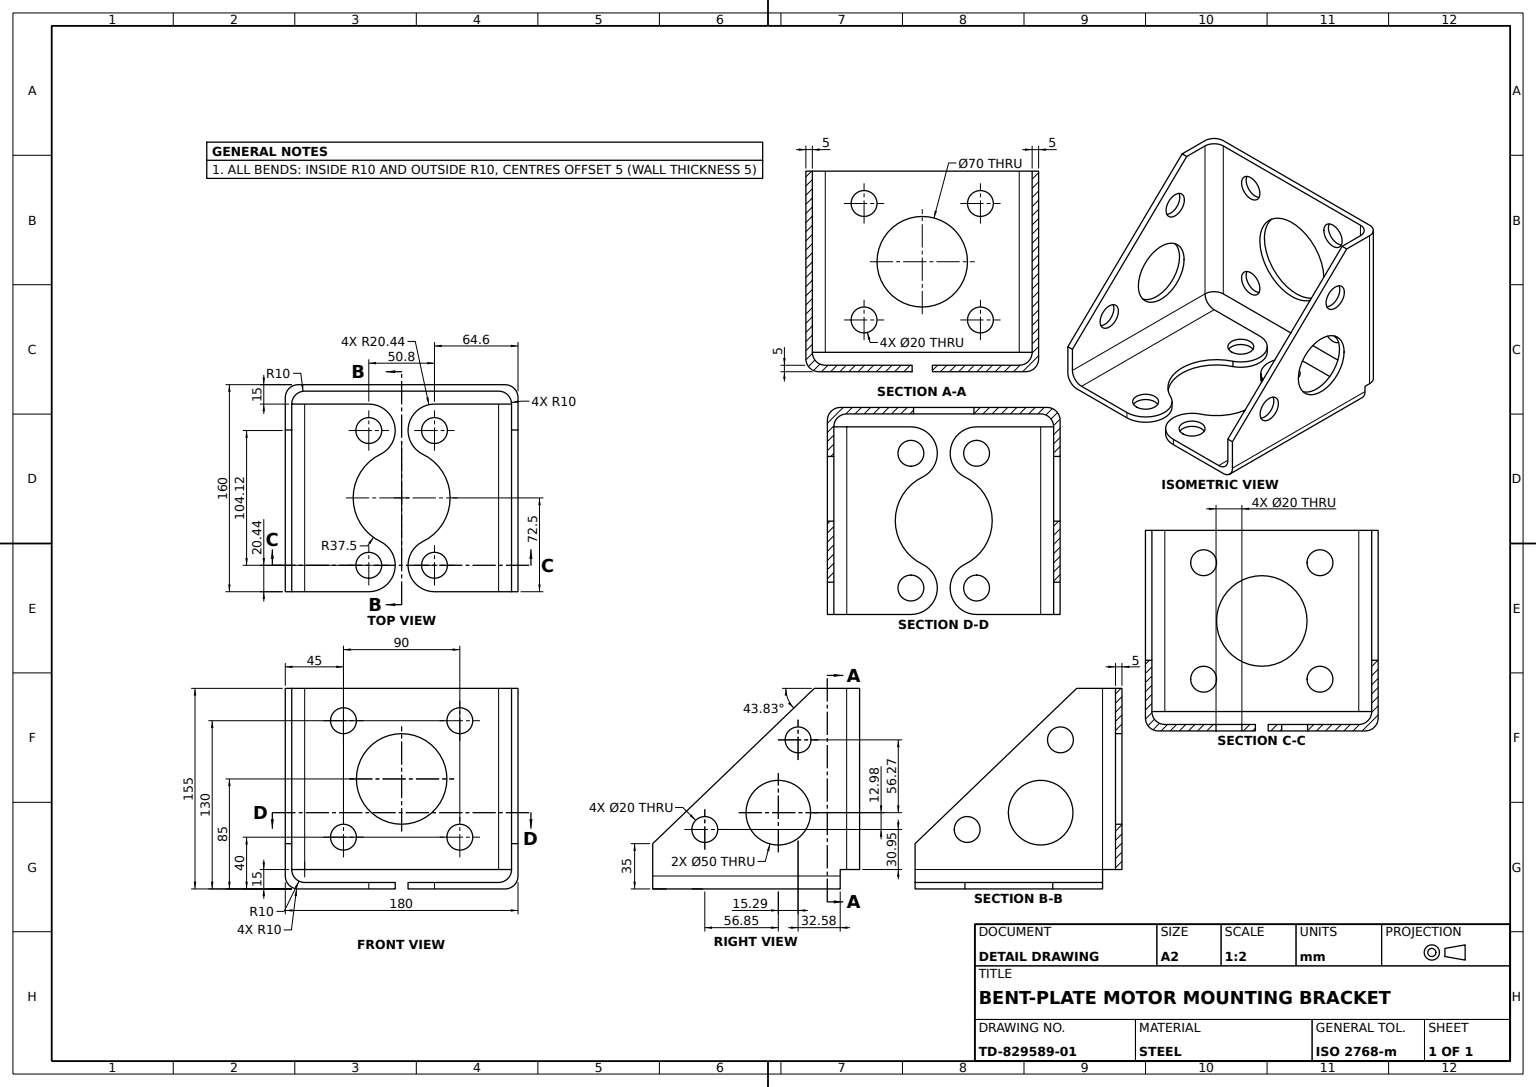
from build123d import *

# Parameters (mm, degrees)
BASE_FLANGE_SKETCH_W     = 180
BASE_FLANGE_SKETCH_H     = 140
BASE_FLANGE_SKETCH_R     = 35
BASE_FLANGE_SKETCH_R_2   = 10
BASE_FLANGE_5MM_DEPTH    = 5
SIDE_GUSSET_SKETCH_R     = 25
SIDE_GUSSET_SKETCH_R_2   = 10
SIDE_GUSSET_SKETCH_W     = 5
SIDE_GUSSET_SKETCH_H     = 140
SIDE_GUSSET_A_DEPTH      = 5
SIDE_START               = -175
SKETCH2_5_R              = 25
SKETCH2_5_R_2            = 10
SKETCH2_5_W              = 5
SKETCH2_5_H              = 140
SIDE_GUSSET_B_DEPTH      = 5
BASE_FLANGE_FILLET_R10_R = 10
GUSSET_EDGE_FILLET_R10_R = 10
BACK_PLATE_SKETCH_W      = 5
BACK_PLATE_SKETCH_H      = 145
BACK_PLATE_DEPTH         = 15
MOTOR_MOUNT_PAD_SKETCH_R = 10
MOTOR_MOUNT_PAD_SKETCH_W = 5
MOTOR_MOUNT_PAD_SKETCH_H = 145
MOTOR_MOUNT_PAD_DEPTH    = 5
MOUNT_EDGE_FILLET_R10_R  = 10


with BuildPart() as part:
    # Base Flange Sketch → Base Flange 5mm (new body)
    with BuildSketch(Plane.XY):
        Rectangle(BASE_FLANGE_SKETCH_W, BASE_FLANGE_SKETCH_H)
        Circle(BASE_FLANGE_SKETCH_R, mode=Mode.SUBTRACT)
        with Locations((-45, 45)):
            Circle(BASE_FLANGE_SKETCH_R_2, mode=Mode.SUBTRACT)
        with Locations((45, 45)):
            Circle(BASE_FLANGE_SKETCH_R_2, mode=Mode.SUBTRACT)
        with Locations((-45, -45)):
            Circle(BASE_FLANGE_SKETCH_R_2, mode=Mode.SUBTRACT)
        with Locations((45, -45)):
            Circle(BASE_FLANGE_SKETCH_R_2, mode=Mode.SUBTRACT)
    extrude(amount=BASE_FLANGE_5MM_DEPTH)

    # Side Gusset Sketch → Side Gusset A (add)
    # profile 1 of 2: a face of its own
    with BuildSketch(Plane.ZY.offset(90)):
        Polygon((35, 70), (5, 70), (5, -70), (160, -70), (160, -50), (133.569366052, -24.626591409), (97.5, 10), (61.430633948, 44.626591409), align=None)
        with Locations((62.873408591, -26.069366052)):
            Circle(SIDE_GUSSET_SKETCH_R, mode=Mode.SUBTRACT)
        with Locations((119.718729488, -39.05433783)):
            Circle(SIDE_GUSSET_SKETCH_R_2, mode=Mode.SUBTRACT)
        with Locations((47.579997385, 30.198844989)):
            Circle(SIDE_GUSSET_SKETCH_R_2, mode=Mode.SUBTRACT)
    # profile 2 of 2: a face of its own
    with BuildSketch(Plane.ZY.offset(90)):
        with Locations((2.5, 0)):
            Rectangle(SIDE_GUSSET_SKETCH_W, SIDE_GUSSET_SKETCH_H)
    extrude(amount=-SIDE_GUSSET_A_DEPTH)

    # Sketch2_5 → Side Gusset B (add)
    # profile 1 of 2: a face of its own
    with BuildSketch(Plane.ZY.offset(90).offset(SIDE_START)):
        Polygon((35, 70), (5, 70), (5, -70), (160, -70), (160, -50), (133.569366052, -24.626591409), (97.5, 10), (61.430633948, 44.626591409), align=None)
        with Locations((62.873408591, -26.069366052)):
            Circle(SKETCH2_5_R, mode=Mode.SUBTRACT)
        with Locations((119.718729488, -39.05433783)):
            Circle(SKETCH2_5_R_2, mode=Mode.SUBTRACT)
        with Locations((47.579997385, 30.198844989)):
            Circle(SKETCH2_5_R_2, mode=Mode.SUBTRACT)
    # profile 2 of 2: a face of its own
    with BuildSketch(Plane.ZY.offset(90).offset(SIDE_START)):
        with Locations((2.5, 0)):
            Rectangle(SKETCH2_5_W, SKETCH2_5_H)
    extrude(amount=-SIDE_GUSSET_B_DEPTH)

    # Base Flange Fillet R10
    base_flange_fillet_r10_edges = [part.edges().sort_by_distance(p)[0] for p in [
        (-90, 0, 0),
        (90, 0, 0),
    ]]
    fillet(base_flange_fillet_r10_edges, radius=BASE_FLANGE_FILLET_R10_R)

    # Gusset Edge Fillet R10
    gusset_edge_fillet_r10_edges = [part.edges().sort_by_distance(p)[0] for p in [
        (-85, 0, 5),
        (85, 0, 5),
    ]]
    fillet(gusset_edge_fillet_r10_edges, radius=GUSSET_EDGE_FILLET_R10_R)

    # Back Plate Sketch → Back Plate (add)
    with BuildSketch(Plane.XZ.offset(70)):
        with Locations((-87.5, 87.5)):
            Rectangle(BACK_PLATE_SKETCH_W, BACK_PLATE_SKETCH_H)
        with Locations((87.5, 87.5)):
            Rectangle(BACK_PLATE_SKETCH_W, BACK_PLATE_SKETCH_H)
    extrude(amount=BACK_PLATE_DEPTH)

    # Motor Mount Pad Sketch → Motor Mount Pad (add)
    # profile 1 of 3: a face of its own
    with BuildSketch(Plane.XZ.offset(85)):
        with BuildLine():
            Line((-25.4, 160), (-85, 160))
            Line((-85, 160), (-85, 15))
            Line((-85, 15), (-25.4, 15))
            ThreePointArc((-25.4, 15), (-5.555268835, 30.543037168), (-15.891300301, 53.533596382))
            ThreePointArc((-15.891300301, 53.533596382), (-16.443437096, 53.797427747), (-16.991195266, 54.070233572))
            ThreePointArc((-16.991195266, 54.070233572), (-37.5, 87.5), (-16.991195266, 120.929766428))
            ThreePointArc((-16.991195266, 120.929766428), (-16.443437096, 121.202572253), (-15.891300301, 121.466403618))
            ThreePointArc((-15.891300301, 121.466403618), (-5.555268835, 144.456962832), (-25.4, 160))
        make_face()
        with Locations(Location((-25.4, 35.44, 0), (0, 0, 270))):
            Circle(MOTOR_MOUNT_PAD_SKETCH_R, mode=Mode.SUBTRACT)
        with Locations(Location((-25.4, 139.56, 0), (0, 0, 270))):
            Circle(MOTOR_MOUNT_PAD_SKETCH_R, mode=Mode.SUBTRACT)
    # profile 2 of 3: a face of its own
    with BuildSketch(Plane.XZ.offset(85)):
        with BuildLine():
            Line((90, 160), (25.4, 160))
            ThreePointArc((25.4, 160), (5.555268835, 144.456962832), (15.891300301, 121.466403618))
            ThreePointArc((15.891300301, 121.466403618), (16.443437096, 121.202572253), (16.991195266, 120.929766428))
            ThreePointArc((16.991195266, 120.929766428), (37.5, 87.5), (16.991195266, 54.070233572))
            ThreePointArc((16.991195266, 54.070233572), (16.443437096, 53.797427747), (15.891300301, 53.533596382))
            ThreePointArc((15.891300301, 53.533596382), (5.555268835, 30.543037168), (25.4, 15))
            Line((25.4, 15), (90, 15))
            Line((90, 15), (90, 160))
        make_face()
        with Locations(Location((25.4, 35.44, 0), (0, 0, 270))):
            Circle(MOTOR_MOUNT_PAD_SKETCH_R, mode=Mode.SUBTRACT)
        with Locations(Location((25.4, 139.56, 0), (0, 0, 270))):
            Circle(MOTOR_MOUNT_PAD_SKETCH_R, mode=Mode.SUBTRACT)
    # profile 3 of 3: a face of its own
    with BuildSketch(Plane.XZ.offset(85)):
        with Locations((-87.5, 87.5)):
            Rectangle(MOTOR_MOUNT_PAD_SKETCH_W, MOTOR_MOUNT_PAD_SKETCH_H)
    extrude(amount=-MOTOR_MOUNT_PAD_DEPTH)

    # Mount Edge Fillet R10
    mount_edge_fillet_r10_edges = [part.edges().sort_by_distance(p)[0] for p in [
        (85, -80, 87.5),
        (90, -85, 87.5),
        (-90, -85, 87.5),
        (-85, -80, 87.5),
    ]]
    fillet(mount_edge_fillet_r10_edges, radius=MOUNT_EDGE_FILLET_R10_R)


solid = part.part
